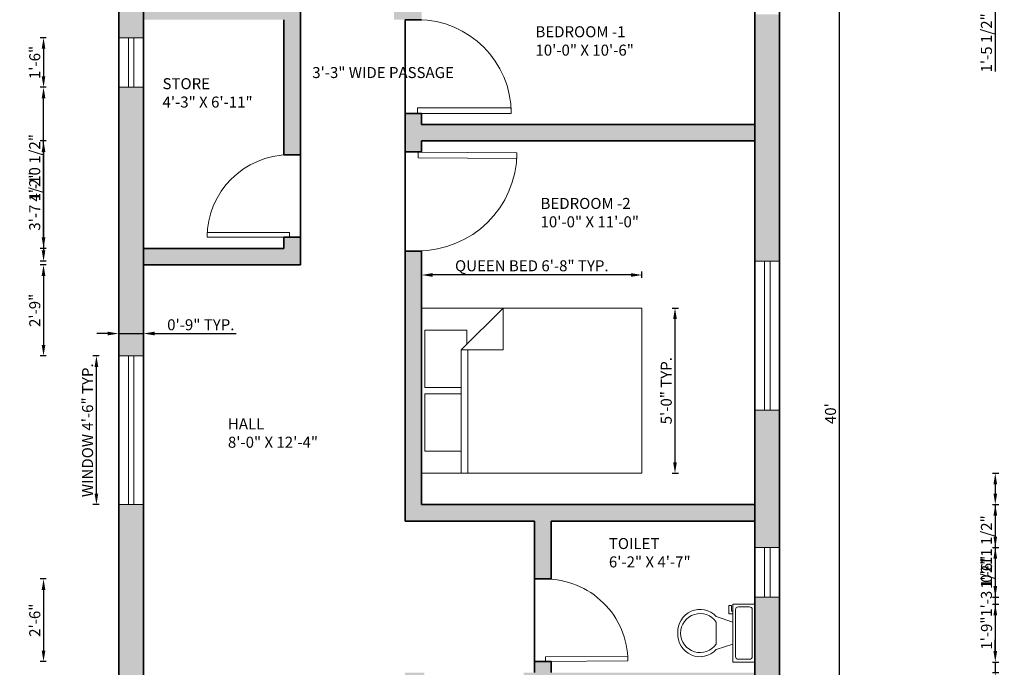
# Model space of a CAD drawing. Units: inches. Extents: x -35 to 322, y -513 to 50.
# Tile 2 of 3: x -35 to 322, y -318 to -83. Entities that reach past the tile are written whole.
import ezdxf

# ---------------------------------------------------------------- set-up
doc = ezdxf.new("R2010")
doc.units = ezdxf.units.IN
for name, color, linetype, lineweight in [('A-ANNO-DIMS', 2, 'Continuous', 18), ('A-AREA-IDEN', 7, 'Continuous', 18), ('A-DOOR', 4, 'Continuous', 18), ('A-FLOR-FIXT', 9, 'Continuous', 18), ('A-FURN', 8, 'Continuous', 18), ('A-GLAZ', 6, 'Continuous', 18), ('A-WALL', 7, 'Continuous', 35), ('A-WALL-PATT', 251, 'Continuous', 13)]:
    doc.layers.add(name, color=color, linetype=linetype, lineweight=lineweight)
doc.styles.get("Standard").update_dxf_attribs({"font": 'arial.ttf'})
doc.dimstyles.new('ISO-25', dxfattribs={"dimtxt": 4, "dimasz": 4, "dimexe": 1.25, "dimexo": 0.625, "dimtad": 1, "dimlunit": 3, "dimtxsty": 'Standard', "dimcen": 2.5, "dimadec": 0, "dimazin": 0, "dimtfac": 1, "dimtmove": 0, "dimatfit": 3, "dimfxl": 1, "dimfxlon": 1, "dimarcsym": 0})

# ---------------------------------------------------------------- blocks, each defined once
blk = doc.blocks.new('*U2')
for p, q in [((9.5, -6), (9.5, -2)), ((-10, -8.5), (-8, -8.5)), ((-10, -9.5), (-10, -8.5)), ((-7, -9.5), (-10, -9.5)), ((-8, -8.5), (-8, -8)), ((-7, -8), (-7, -9.5)), ((-4, -8), (-6, -14)), ((4, -8), (6, -14)), ((4, -14), (-4, -14))]:
    blk.add_line(p, q)
blk.add_lwpolyline([(10.5, -8), (10.5, 0), (-10.5, 0), (-10.5, -8)], close=True)
for points in [[(-9.5, -2), (-9.5, -6)], [(8.5, -1), (-8.5, -1)], [(-8.5, -7), (8.5, -7)]]:
    blk.add_lwpolyline(points)
for centre, radius, start, end in [((-8.625, -1.875), 0.8839, 81.8699, 188.1301), ((8.625, -1.875), 0.8839, 351.8699, 98.1301), ((-8.625, -6.125), 0.8839, 171.869898, 278.1301), ((8.625, -6.125), 0.8839, 261.8699, 8.1301), ((-0.4772, -19.9188), 8.0953, 133.01722, 273.38), ((0.0374, -19.8731), 7.127, 124.50543, 269.7), ((-0.0373, -19.8731), 7.127, 270.3, 55.4946), ((0.4773, -19.9188), 8.0953, 266.62, 46.9828)]:
    blk.add_arc(centre, radius, start, end)
blk = doc.blocks.new('*U4')
for p, q in [((0, 0), (0, -100)), ((750, 0), (750, -100))]:
    blk.add_line(p, q)
blk.add_lwpolyline([(0, 0), (0, 750), (43.75, 750), (43.75, 0)], close=True)
blk.add_arc((0, 0), 750, 0, 90)
blk = doc.blocks.new('Bed - Queen')
for p, q in [((0, -80.00003), (0, 0)), ((0, 0), (59.99999, 0)), ((59.99999, 0), (59.99999, -80.00003)), ((7.99999, -1.2), (28.79998, -1.2)), ((7.99999, -14.4), (7.99999, -1.2)), ((28.79998, -1.2), (28.79998, -14.4)), ((31.19999, -1.2), (51.99999, -1.2)), ((31.19999, -14.4), (31.19999, -1.2)), ((51.99999, -1.2), (51.99999, -16.4)), ((0, -14.4), (44.8, -14.4)), ((44.8, -16.8), (0, -16.8)), ((59.99999, -29.6), (44.8, -14.4)), ((44.8, -14.4), (44.8, -29.6)), ((51.99999, -16.4), (46.79936, -16.4)), ((44.8, -29.6), (59.99999, -29.6)), ((59.99999, -80.00003), (0, -80.00003))]:
    blk.add_line(p, q)
blk = doc.blocks.new('*D13')
at = {"layer": 'A-ANNO-DIMS', "color": 0, "lineweight": -2, "transparency": 16777216}
for p, q in [((261.29, 13.99), (263.54, 13.99)), ((262.29, 9.99), (262.29, -462.01)), ((261.29, -466.01), (263.54, -466.01))]:
    blk.add_line(p, q, dxfattribs=at)
at = {"layer": 'A-ANNO-DIMS', "color": 0, "transparency": 16777216}
for points in [[(261.62, 9.99), (262.95, 9.99), (262.29, 13.99)], [(261.62, -462.01), (262.95, -462.01), (262.29, -466.01)]]:
    blk.add_solid(points, dxfattribs=at)
at = {"layer": 'Defpoints', "color": 0, "transparency": 16777216}
for p in [(239.43, 13.99), (240.64, -466.01), (262.29, -466.01)]:
    blk.add_point(p, dxfattribs=at)
at = {"layer": 'A-ANNO-DIMS', "color": 0, "transparency": 16777216, "insert": (259.62, -226.01), "char_height": 4, "attachment_point": 5, "rotation": 90}
blk.add_mtext("40'", dxfattribs=at)
blk = doc.blocks.new('WIN-54IN')
for p, q in [((3.5, 54), (3.5, 0)), ((5.5, 54), (5.5, 0))]:
    blk.add_line(p, q)
blk.add_lwpolyline([(0, 54), (9, 54), (9, 0), (0, 0)], close=True)
blk = doc.blocks.new('*D16')
at = {"layer": 'A-ANNO-DIMS', "color": 0, "lineweight": -2, "transparency": 16777216}
for p, q in [((110.64, -176.68), (110.64, -174.43)), ((190.64, -176.68), (190.64, -174.43)), ((186.64, -175.68), (114.64, -175.68))]:
    blk.add_line(p, q, dxfattribs=at)
at = {"layer": 'A-ANNO-DIMS', "color": 0, "transparency": 16777216}
for points in [[(114.64, -175.01), (114.64, -176.35), (110.64, -175.68)], [(186.64, -175.01), (186.64, -176.35), (190.64, -175.68)]]:
    blk.add_solid(points, dxfattribs=at)
at = {"layer": 'Defpoints', "color": 0, "transparency": 16777216}
for p in [(110.64, -175.68), (110.64, -187.68), (190.64, -187.68)]:
    blk.add_point(p, dxfattribs=at)
at = {"layer": 'A-ANNO-DIMS', "color": 0, "transparency": 16777216, "insert": (150.64, -172.86), "char_height": 4, "attachment_point": 5}
blk.add_mtext('QUEEN BED 6\'-8" TYP.', dxfattribs=at)
blk = doc.blocks.new('*D17')
at = {"layer": 'A-ANNO-DIMS', "color": 0, "lineweight": -2, "transparency": 16777216}
for p, q in [((201.64, -187.68), (203.89, -187.68)), ((202.64, -243.68), (202.64, -191.68)), ((201.64, -247.68), (203.89, -247.68))]:
    blk.add_line(p, q, dxfattribs=at)
at = {"layer": 'A-ANNO-DIMS', "color": 0, "transparency": 16777216}
for points in [[(201.97, -191.68), (203.3, -191.68), (202.64, -187.68)], [(201.97, -243.68), (203.3, -243.68), (202.64, -247.68)]]:
    blk.add_solid(points, dxfattribs=at)
at = {"layer": 'Defpoints', "color": 0, "transparency": 16777216}
for p in [(190.64, -187.68), (202.64, -187.68), (190.64, -247.68)]:
    blk.add_point(p, dxfattribs=at)
at = {"layer": 'A-ANNO-DIMS', "color": 0, "transparency": 16777216, "insert": (199.97, -217.68), "char_height": 4, "attachment_point": 5, "rotation": 90}
blk.add_mtext('5\'-0" TYP.', dxfattribs=at)
blk = doc.blocks.new('*D18')
at = {"layer": 'A-ANNO-DIMS', "color": 0, "lineweight": -2, "transparency": 16777216}
for p, q in [((-6.46, -205.04), (-8.71, -205.04)), ((-7.46, -255.04), (-7.46, -209.04)), ((-6.46, -259.04), (-8.71, -259.04))]:
    blk.add_line(p, q, dxfattribs=at)
at = {"layer": 'A-ANNO-DIMS', "color": 0, "transparency": 16777216}
for points in [[(-8.13, -209.04), (-6.8, -209.04), (-7.46, -205.04)], [(-8.13, -255.04), (-6.8, -255.04), (-7.46, -259.04)]]:
    blk.add_solid(points, dxfattribs=at)
at = {"layer": 'Defpoints', "color": 0, "transparency": 16777216}
for p in [(-7.46, -205.04), (0.64, -205.04), (0.64, -259.04)]:
    blk.add_point(p, dxfattribs=at)
at = {"layer": 'A-ANNO-DIMS', "color": 0, "transparency": 16777216, "insert": (-10.16, -232.04), "char_height": 4, "attachment_point": 5, "rotation": 90}
blk.add_mtext('WINDOW 4\'-6" TYP.', dxfattribs=at)
blk = doc.blocks.new('*D19')
at = {"layer": 'A-ANNO-DIMS', "color": 0, "lineweight": -2, "transparency": 16777216}
for p, q in [((0.64, -197.94), (0.64, -195.69)), ((9.64, -197.94), (9.64, -195.69)), ((-3.36, -196.94), (-7.36, -196.94)), ((0.64, -196.94), (9.64, -196.94)), ((13.64, -196.94), (43.27, -196.94))]:
    blk.add_line(p, q, dxfattribs=at)
at = {"layer": 'A-ANNO-DIMS', "color": 0, "transparency": 16777216}
for points in [[(-3.36, -196.27), (-3.36, -197.61), (0.64, -196.94)], [(13.64, -196.27), (13.64, -197.61), (9.64, -196.94)]]:
    blk.add_solid(points, dxfattribs=at)
at = {"layer": 'Defpoints', "color": 0, "transparency": 16777216}
for p in [(9.64, -196.94), (0.64, -205.04), (9.64, -205.04)]:
    blk.add_point(p, dxfattribs=at)
at = {"layer": 'A-ANNO-DIMS', "color": 0, "transparency": 16777216, "insert": (30.45, -194.27), "char_height": 4, "attachment_point": 5}
blk.add_mtext('0\'-9" TYP.', dxfattribs=at)
blk = doc.blocks.new('*D26')
at = {"layer": 'A-ANNO-DIMS', "color": 0, "lineweight": -2, "transparency": 16777216}
for p, q in [((100.64, -509.7), (96.64, -509.7)), ((104.64, -508.7), (104.64, -510.95)), ((104.64, -509.7), (110.64, -509.7)), ((110.64, -508.7), (110.64, -510.95)), ((114.64, -509.7), (130.52, -509.7))]:
    blk.add_line(p, q, dxfattribs=at)
at = {"layer": 'A-ANNO-DIMS', "color": 0, "transparency": 16777216}
for points in [[(100.64, -509.04), (100.64, -510.37), (104.64, -509.7)], [(114.64, -509.04), (114.64, -510.37), (110.64, -509.7)]]:
    blk.add_solid(points, dxfattribs=at)
at = {"layer": 'Defpoints', "color": 0, "transparency": 16777216}
for p in [(104.64, -77.01), (110.64, -83.01), (110.64, -509.7)]:
    blk.add_point(p, dxfattribs=at)
at = {"layer": 'A-ANNO-DIMS', "color": 0, "transparency": 16777216, "insert": (124.58, -507.04), "char_height": 4, "attachment_point": 5}
blk.add_mtext('0\'-6"', dxfattribs=at)
blk = doc.blocks.new('*D29')
at = {"layer": 'A-ANNO-DIMS', "color": 0, "lineweight": -2, "transparency": 16777216}
for p, q in [((66.64, 40.29), (66.64, 42.54)), ((70.64, 41.29), (100.64, 41.29)), ((104.64, 40.29), (104.64, 42.54))]:
    blk.add_line(p, q, dxfattribs=at)
at = {"layer": 'A-ANNO-DIMS', "color": 0, "transparency": 16777216}
for points in [[(70.64, 41.95), (70.64, 40.62), (66.64, 41.29)], [(100.64, 41.95), (100.64, 40.62), (104.64, 41.29)]]:
    blk.add_solid(points, dxfattribs=at)
at = {"layer": 'Defpoints', "color": 0, "transparency": 16777216}
for p in [(104.64, 41.29), (66.64, -466.01), (104.64, -466.01)]:
    blk.add_point(p, dxfattribs=at)
at = {"layer": 'A-ANNO-DIMS', "color": 0, "transparency": 16777216, "insert": (85.64, 43.96), "char_height": 4, "attachment_point": 5}
blk.add_mtext('3\'-2"', dxfattribs=at)
blk = doc.blocks.new('*D35')
at = {"layer": 'A-ANNO-DIMS', "color": 0, "lineweight": -2, "transparency": 16777216}
for p, q in [((-25.66, -107.55), (-27.91, -107.55)), ((-26.66, -162.01), (-26.66, -111.55)), ((-25.66, -166.01), (-27.91, -166.01))]:
    blk.add_line(p, q, dxfattribs=at)
at = {"layer": 'A-ANNO-DIMS', "color": 0, "transparency": 16777216}
for points in [[(-27.33, -111.55), (-26, -111.55), (-26.66, -107.55)], [(-27.33, -162.01), (-26, -162.01), (-26.66, -166.01)]]:
    blk.add_solid(points, dxfattribs=at)
at = {"layer": 'Defpoints', "color": 0, "transparency": 16777216}
for p in [(-26.66, -107.55), (9.64, -107.55), (9.64, -166.01)]:
    blk.add_point(p, dxfattribs=at)
at = {"layer": 'A-ANNO-DIMS', "color": 0, "transparency": 16777216, "insert": (-29.36, -136.78), "char_height": 4, "attachment_point": 5, "rotation": 90}
blk.add_mtext('4\'-10 1/2"', dxfattribs=at)
blk = doc.blocks.new('*D36')
at = {"layer": 'A-ANNO-DIMS', "color": 0, "lineweight": -2, "transparency": 16777216}
for p, q in [((-25.66, -89.55), (-27.91, -89.55)), ((-26.66, -93.55), (-26.66, -103.55)), ((-25.66, -107.55), (-27.91, -107.55))]:
    blk.add_line(p, q, dxfattribs=at)
at = {"layer": 'A-ANNO-DIMS', "color": 0, "transparency": 16777216}
for points in [[(-27.33, -93.55), (-26, -93.55), (-26.66, -89.55)], [(-27.33, -103.55), (-26, -103.55), (-26.66, -107.55)]]:
    blk.add_solid(points, dxfattribs=at)
at = {"layer": 'Defpoints', "color": 0, "transparency": 16777216}
for p in [(0.64, -89.55), (-26.66, -107.55), (0.64, -107.55)]:
    blk.add_point(p, dxfattribs=at)
at = {"layer": 'A-ANNO-DIMS', "color": 0, "transparency": 16777216, "insert": (-29.33, -98.55), "char_height": 4, "attachment_point": 5, "rotation": 90}
blk.add_mtext('1\'-6"', dxfattribs=at)
blk = doc.blocks.new('*D37')
at = {"layer": 'A-ANNO-DIMS', "color": 0, "lineweight": -2, "transparency": 16777216}
for p, q in [((-25.66, -172.01), (-27.91, -172.01)), ((-26.66, -176.01), (-26.66, -201.04)), ((-25.66, -205.04), (-27.91, -205.04))]:
    blk.add_line(p, q, dxfattribs=at)
at = {"layer": 'A-ANNO-DIMS', "color": 0, "transparency": 16777216}
for points in [[(-27.33, -176.01), (-26, -176.01), (-26.66, -172.01)], [(-27.33, -201.04), (-26, -201.04), (-26.66, -205.04)]]:
    blk.add_solid(points, dxfattribs=at)
at = {"layer": 'Defpoints', "color": 0, "transparency": 16777216}
for p in [(9.64, -172.01), (-26.66, -205.04), (9.64, -205.04)]:
    blk.add_point(p, dxfattribs=at)
at = {"layer": 'A-ANNO-DIMS', "color": 0, "transparency": 16777216, "insert": (-29.33, -188.53), "char_height": 4, "attachment_point": 5, "rotation": 90}
blk.add_mtext('2\'-9"', dxfattribs=at)
blk = doc.blocks.new('*D39')
at = {"layer": 'A-ANNO-DIMS', "color": 0, "lineweight": -2, "transparency": 16777216}
for p, q in [((-25.66, -127.01), (-27.91, -127.01)), ((-26.66, -131.01), (-26.66, -166.72)), ((-25.66, -170.72), (-27.91, -170.72))]:
    blk.add_line(p, q, dxfattribs=at)
at = {"layer": 'A-ANNO-DIMS', "color": 0, "transparency": 16777216}
for points in [[(-27.33, -131.01), (-26, -131.01), (-26.66, -127.01)], [(-27.33, -166.72), (-26, -166.72), (-26.66, -170.72)]]:
    blk.add_solid(points, dxfattribs=at)
at = {"layer": 'Defpoints', "color": 0, "transparency": 16777216}
for p in [(231.64, -127.01), (-26.66, -170.72), (231.64, -170.72)]:
    blk.add_point(p, dxfattribs=at)
at = {"layer": 'A-ANNO-DIMS', "color": 0, "transparency": 16777216, "insert": (-29.36, -148.86), "char_height": 4, "attachment_point": 5, "rotation": 90}
blk.add_mtext('3\'-7 1/2"', dxfattribs=at)
blk = doc.blocks.new('*D40')
at = {"layer": 'A-ANNO-DIMS', "color": 0, "lineweight": -2, "transparency": 16777216}
for p, q in [((317.94, -259.01), (320.19, -259.01)), ((318.94, -263.01), (318.94, -270.62)), ((317.94, -274.62), (320.19, -274.62)), ((318.94, -274.62), (318.94, -299.45))]:
    blk.add_line(p, q, dxfattribs=at)
at = {"layer": 'A-ANNO-DIMS', "color": 0, "transparency": 16777216}
for points in [[(318.27, -263.01), (319.6, -263.01), (318.94, -259.01)], [(318.27, -270.62), (319.6, -270.62), (318.94, -274.62)]]:
    blk.add_solid(points, dxfattribs=at)
at = {"layer": 'Defpoints', "color": 0, "transparency": 16777216}
for p in [(231.64, -259.01), (240.64, -274.62), (318.94, -274.62)]:
    blk.add_point(p, dxfattribs=at)
at = {"layer": 'A-ANNO-DIMS', "color": 0, "transparency": 16777216, "insert": (316.24, -289.04), "char_height": 4, "attachment_point": 5, "rotation": 90}
blk.add_mtext('1\'-3 1/2"', dxfattribs=at)
blk = doc.blocks.new('*D41')
at = {"layer": 'A-ANNO-DIMS', "color": 0, "lineweight": -2, "transparency": 16777216}
for p, q in [((317.94, -274.62), (320.19, -274.62)), ((318.94, -278.62), (318.94, -288.62)), ((317.94, -292.62), (320.19, -292.62))]:
    blk.add_line(p, q, dxfattribs=at)
at = {"layer": 'A-ANNO-DIMS', "color": 0, "transparency": 16777216}
for points in [[(318.27, -278.62), (319.6, -278.62), (318.94, -274.62)], [(318.27, -288.62), (319.6, -288.62), (318.94, -292.62)]]:
    blk.add_solid(points, dxfattribs=at)
at = {"layer": 'Defpoints', "color": 0, "transparency": 16777216}
for p in [(240.64, -274.62), (240.64, -292.62), (318.94, -292.62)]:
    blk.add_point(p, dxfattribs=at)
at = {"layer": 'A-ANNO-DIMS', "color": 0, "transparency": 16777216, "insert": (316.27, -283.62), "char_height": 4, "attachment_point": 5, "rotation": 90}
blk.add_mtext('1\'-6"', dxfattribs=at)
blk = doc.blocks.new('*D42')
at = {"layer": 'A-ANNO-DIMS', "color": 0, "lineweight": -2, "transparency": 16777216}
for p, q in [((196.08, 40.29), (196.08, 42.54)), ((200.08, 41.29), (227.64, 41.29)), ((231.64, 40.29), (231.64, 42.54))]:
    blk.add_line(p, q, dxfattribs=at)
at = {"layer": 'A-ANNO-DIMS', "color": 0, "transparency": 16777216}
for points in [[(200.08, 41.95), (200.08, 40.62), (196.08, 41.29)], [(227.64, 41.95), (227.64, 40.62), (231.64, 41.29)]]:
    blk.add_solid(points, dxfattribs=at)
at = {"layer": 'Defpoints', "color": 0, "transparency": 16777216}
for p in [(231.64, 41.29), (196.08, -457.01), (231.64, -457.01)]:
    blk.add_point(p, dxfattribs=at)
at = {"layer": 'A-ANNO-DIMS', "color": 0, "transparency": 16777216, "insert": (213.86, 43.98), "char_height": 4, "attachment_point": 5}
blk.add_mtext('2\'-11 1/2"', dxfattribs=at)
blk = doc.blocks.new('*D43')
at = {"layer": 'A-ANNO-DIMS', "color": 0, "lineweight": -2, "transparency": 16777216}
for p, q in [((66.64, -508.7), (66.64, -510.95)), ((70.64, -509.7), (96.64, -509.7)), ((100.64, -508.7), (100.64, -510.95))]:
    blk.add_line(p, q, dxfattribs=at)
at = {"layer": 'A-ANNO-DIMS', "color": 0, "transparency": 16777216}
for points in [[(70.64, -509.04), (70.64, -510.37), (66.64, -509.7)], [(96.64, -509.04), (96.64, -510.37), (100.64, -509.7)]]:
    blk.add_solid(points, dxfattribs=at)
at = {"layer": 'Defpoints', "color": 0, "transparency": 16777216}
for p in [(66.64, -83.01), (100.64, -83.01), (100.64, -509.7)]:
    blk.add_point(p, dxfattribs=at)
at = {"layer": 'A-ANNO-DIMS', "color": 0, "transparency": 16777216, "insert": (83.64, -507.04), "char_height": 4, "attachment_point": 5}
blk.add_mtext('2\'-10"', dxfattribs=at)
blk = doc.blocks.new('*D46')
at = {"layer": 'A-ANNO-DIMS', "color": 0, "lineweight": -2, "transparency": 16777216}
for p, q in [((32.73, 40.29), (32.73, 42.54)), ((36.73, 41.29), (58.65, 41.29)), ((62.65, 40.29), (62.65, 42.54))]:
    blk.add_line(p, q, dxfattribs=at)
at = {"layer": 'A-ANNO-DIMS', "color": 0, "transparency": 16777216}
for points in [[(36.73, 41.95), (36.73, 40.62), (32.73, 41.29)], [(58.65, 41.95), (58.65, 40.62), (62.65, 41.29)]]:
    blk.add_solid(points, dxfattribs=at)
at = {"layer": 'Defpoints', "color": 0, "transparency": 16777216}
for p in [(62.65, 41.29), (32.73, -162.01), (62.65, -162.01)]:
    blk.add_point(p, dxfattribs=at)
at = {"layer": 'A-ANNO-DIMS', "color": 0, "transparency": 16777216, "insert": (47.69, 43.95), "char_height": 4, "attachment_point": 5}
blk.add_mtext('2\'-6"', dxfattribs=at)
blk = doc.blocks.new('*D47')
at = {"layer": 'A-ANNO-DIMS', "color": 0, "lineweight": -2, "transparency": 16777216}
for p, q in [((109.17, 40.29), (109.17, 42.54)), ((113.17, 41.29), (139.16, 41.29)), ((143.16, 40.29), (143.16, 42.54))]:
    blk.add_line(p, q, dxfattribs=at)
at = {"layer": 'A-ANNO-DIMS', "color": 0, "transparency": 16777216}
for points in [[(113.17, 41.95), (113.17, 40.62), (109.17, 41.29)], [(139.16, 41.95), (139.16, 40.62), (143.16, 41.29)]]:
    blk.add_solid(points, dxfattribs=at)
at = {"layer": 'Defpoints', "color": 0, "transparency": 16777216}
for p in [(143.16, 41.29), (109.17, -117.01), (143.16, -117.01)]:
    blk.add_point(p, dxfattribs=at)
at = {"layer": 'A-ANNO-DIMS', "color": 0, "transparency": 16777216, "insert": (126.17, 43.95), "char_height": 4, "attachment_point": 5}
blk.add_mtext('2\'-10"', dxfattribs=at)
blk = doc.blocks.new('*D48')
at = {"layer": 'A-ANNO-DIMS', "color": 0, "lineweight": -2, "transparency": 16777216}
for p, q in [((109.42, -508.7), (109.42, -510.95)), ((113.42, -509.7), (141.25, -509.7)), ((145.25, -508.7), (145.25, -510.95))]:
    blk.add_line(p, q, dxfattribs=at)
at = {"layer": 'A-ANNO-DIMS', "color": 0, "transparency": 16777216}
for points in [[(113.42, -509.04), (113.42, -510.37), (109.42, -509.7)], [(141.25, -509.04), (141.25, -510.37), (145.25, -509.7)]]:
    blk.add_solid(points, dxfattribs=at)
at = {"layer": 'Defpoints', "color": 0, "transparency": 16777216}
for p in [(109.42, -131.05), (145.25, -131.34), (145.25, -509.7)]:
    blk.add_point(p, dxfattribs=at)
at = {"layer": 'A-ANNO-DIMS', "color": 0, "transparency": 16777216, "insert": (127.34, -507.04), "char_height": 4, "attachment_point": 5}
blk.add_mtext('3\'-0"', dxfattribs=at)
blk = doc.blocks.new('*D49')
at = {"layer": 'A-ANNO-DIMS', "color": 0, "lineweight": -2, "transparency": 16777216}
for p, q in [((-25.66, -286.01), (-27.91, -286.01)), ((-26.66, -290.01), (-26.66, -312.01)), ((-25.66, -316.01), (-27.91, -316.01))]:
    blk.add_line(p, q, dxfattribs=at)
at = {"layer": 'A-ANNO-DIMS', "color": 0, "transparency": 16777216}
for points in [[(-27.33, -290.01), (-26, -290.01), (-26.66, -286.01)], [(-27.33, -312.01), (-26, -312.01), (-26.66, -316.01)]]:
    blk.add_solid(points, dxfattribs=at)
at = {"layer": 'Defpoints', "color": 0, "transparency": 16777216}
for p in [(151.64, -286.01), (-26.66, -316.01), (151.64, -316.01)]:
    blk.add_point(p, dxfattribs=at)
at = {"layer": 'A-ANNO-DIMS', "color": 0, "transparency": 16777216, "insert": (-29.33, -301.01), "char_height": 4, "attachment_point": 5, "rotation": 90}
blk.add_mtext('2\'-6"', dxfattribs=at)
blk = doc.blocks.new('*D50')
at = {"layer": 'A-ANNO-DIMS', "color": 0, "lineweight": -2, "transparency": 16777216}
for p, q in [((111.64, 40.29), (111.64, 42.54)), ((115.64, 41.29), (143.64, 41.29)), ((147.64, 40.29), (147.64, 42.54))]:
    blk.add_line(p, q, dxfattribs=at)
at = {"layer": 'A-ANNO-DIMS', "color": 0, "transparency": 16777216}
for points in [[(115.64, 41.95), (115.64, 40.62), (111.64, 41.29)], [(143.64, 41.95), (143.64, 40.62), (147.64, 41.29)]]:
    blk.add_solid(points, dxfattribs=at)
at = {"layer": 'Defpoints', "color": 0, "transparency": 16777216}
for p in [(147.64, 41.29), (111.64, -320.01), (147.64, -320.01)]:
    blk.add_point(p, dxfattribs=at)
at = {"layer": 'A-ANNO-DIMS', "color": 0, "transparency": 16777216, "insert": (129.64, 43.96), "char_height": 4, "attachment_point": 5}
blk.add_mtext('3\'-0"', dxfattribs=at)
blk = doc.blocks.new('*D51')
at = {"layer": 'A-ANNO-DIMS', "color": 0, "lineweight": -2, "transparency": 16777216}
for p, q in [((203.64, 40.29), (203.64, 42.54)), ((207.64, 41.29), (227.64, 41.29)), ((231.64, 40.29), (231.64, 42.54))]:
    blk.add_line(p, q, dxfattribs=at)
at = {"layer": 'A-ANNO-DIMS', "color": 0, "transparency": 16777216}
for points in [[(207.64, 41.95), (207.64, 40.62), (203.64, 41.29)], [(227.64, 41.95), (227.64, 40.62), (231.64, 41.29)]]:
    blk.add_solid(points, dxfattribs=at)
at = {"layer": 'Defpoints', "color": 0, "transparency": 16777216}
for p in [(231.64, 41.29), (231.64, -295.18), (203.64, -305.68)]:
    blk.add_point(p, dxfattribs=at)
at = {"layer": 'A-ANNO-DIMS', "color": 0, "transparency": 16777216, "insert": (217.64, 43.92), "char_height": 4, "attachment_point": 5}
blk.add_mtext('2\'-4"', dxfattribs=at)
blk = doc.blocks.new('*D52')
at = {"layer": 'A-ANNO-DIMS', "color": 0, "lineweight": -2, "transparency": 16777216}
for p, q in [((317.94, -295.18), (320.19, -295.18)), ((318.94, -299.18), (318.94, -312.18)), ((317.94, -316.18), (320.19, -316.18))]:
    blk.add_line(p, q, dxfattribs=at)
at = {"layer": 'A-ANNO-DIMS', "color": 0, "transparency": 16777216}
for points in [[(318.27, -299.18), (319.6, -299.18), (318.94, -295.18)], [(318.27, -312.18), (319.6, -312.18), (318.94, -316.18)]]:
    blk.add_solid(points, dxfattribs=at)
at = {"layer": 'Defpoints', "color": 0, "transparency": 16777216}
for p in [(231.64, -295.18), (231.64, -316.18), (318.94, -316.18)]:
    blk.add_point(p, dxfattribs=at)
at = {"layer": 'A-ANNO-DIMS', "color": 0, "transparency": 16777216, "insert": (316.27, -305.68), "char_height": 4, "attachment_point": 5, "rotation": 90}
blk.add_mtext('1\'-9"', dxfattribs=at)
blk = doc.blocks.new('*D53')
at = {"layer": 'A-ANNO-DIMS', "color": 0, "lineweight": -2, "transparency": 16777216}
for p, q in [((318.94, -312.18), (318.94, -308.18)), ((317.94, -316.18), (320.19, -316.18)), ((318.94, -316.18), (318.94, -320.01)), ((317.94, -320.01), (320.19, -320.01)), ((318.94, -324.01), (318.94, -339.9))]:
    blk.add_line(p, q, dxfattribs=at)
at = {"layer": 'A-ANNO-DIMS', "color": 0, "transparency": 16777216}
for points in [[(318.27, -312.18), (319.6, -312.18), (318.94, -316.18)], [(318.27, -324.01), (319.6, -324.01), (318.94, -320.01)]]:
    blk.add_solid(points, dxfattribs=at)
at = {"layer": 'Defpoints', "color": 0, "transparency": 16777216}
for p in [(231.64, -316.18), (231.64, -320.01), (318.94, -320.01)]:
    blk.add_point(p, dxfattribs=at)
at = {"layer": 'A-ANNO-DIMS', "color": 0, "transparency": 16777216, "insert": (316.27, -333.95), "char_height": 4, "attachment_point": 5, "rotation": 90}
blk.add_mtext('0\'-4"', dxfattribs=at)
blk = doc.blocks.new('*D54')
at = {"layer": 'A-ANNO-DIMS', "color": 0, "lineweight": -2, "transparency": 16777216}
for p, q in [((209.06, -508.7), (209.06, -510.95)), ((213.06, -509.7), (227.64, -509.7)), ((231.64, -508.7), (231.64, -510.95)), ((231.64, -509.7), (259.57, -509.7))]:
    blk.add_line(p, q, dxfattribs=at)
at = {"layer": 'A-ANNO-DIMS', "color": 0, "transparency": 16777216}
for points in [[(213.06, -509.04), (213.06, -510.37), (209.06, -509.7)], [(227.64, -509.04), (227.64, -510.37), (231.64, -509.7)]]:
    blk.add_solid(points, dxfattribs=at)
at = {"layer": 'Defpoints', "color": 0, "transparency": 16777216}
for p in [(209.06, 4.99), (231.64, 4.99), (231.64, -509.7)]:
    blk.add_point(p, dxfattribs=at)
at = {"layer": 'A-ANNO-DIMS', "color": 0, "transparency": 16777216, "insert": (247.6, -507.01), "char_height": 4, "attachment_point": 5}
blk.add_mtext('1\'-10 1/2"', dxfattribs=at)
blk = doc.blocks.new('*D55')
at = {"layer": 'A-ANNO-DIMS', "color": 0, "lineweight": -2, "transparency": 16777216}
for p, q in [((317.94, -247.68), (320.19, -247.68)), ((318.94, -251.68), (318.94, -255.01)), ((317.94, -259.01), (320.19, -259.01)), ((318.94, -259.01), (318.94, -287.32))]:
    blk.add_line(p, q, dxfattribs=at)
at = {"layer": 'A-ANNO-DIMS', "color": 0, "transparency": 16777216}
for points in [[(318.27, -251.68), (319.6, -251.68), (318.94, -247.68)], [(318.27, -255.01), (319.6, -255.01), (318.94, -259.01)]]:
    blk.add_solid(points, dxfattribs=at)
at = {"layer": 'Defpoints', "color": 0, "transparency": 16777216}
for p in [(190.64, -247.68), (231.64, -259.01), (318.94, -259.01)]:
    blk.add_point(p, dxfattribs=at)
at = {"layer": 'A-ANNO-DIMS', "color": 0, "transparency": 16777216, "insert": (316.24, -275.17), "char_height": 4, "attachment_point": 5, "rotation": 90}
blk.add_mtext('0\'-11 1/2"', dxfattribs=at)
blk = doc.blocks.new('*D59')
at = {"layer": 'A-ANNO-DIMS', "color": 0, "lineweight": -2, "transparency": 16777216}
for p, q in [((317.94, -59.34), (320.19, -59.34)), ((318.94, -63.34), (318.94, -73.01)), ((317.94, -77.01), (320.19, -77.01)), ((318.94, -77.01), (318.94, -101.84))]:
    blk.add_line(p, q, dxfattribs=at)
at = {"layer": 'A-ANNO-DIMS', "color": 0, "transparency": 16777216}
for points in [[(318.27, -63.34), (319.6, -63.34), (318.94, -59.34)], [(318.27, -73.01), (319.6, -73.01), (318.94, -77.01)]]:
    blk.add_solid(points, dxfattribs=at)
at = {"layer": 'Defpoints', "color": 0, "transparency": 16777216}
for p in [(29.69, -59.34), (33.64, -77.01), (318.94, -77.01)]:
    blk.add_point(p, dxfattribs=at)
at = {"layer": 'A-ANNO-DIMS', "color": 0, "transparency": 16777216, "insert": (316.24, -91.43), "char_height": 4, "attachment_point": 5, "rotation": 90}
blk.add_mtext('1\'-5 1/2"', dxfattribs=at)
blk = doc.blocks.new('*D61')
at = {"layer": 'A-ANNO-DIMS', "color": 0, "lineweight": -2, "transparency": 16777216}
for p, q in [((35.64, 41.29), (31.64, 41.29)), ((39.64, 40.29), (39.64, 42.54)), ((39.64, 41.29), (46.39, 41.29)), ((46.39, 40.29), (46.39, 42.54)), ((50.39, 41.29), (66.27, 41.29))]:
    blk.add_line(p, q, dxfattribs=at)
at = {"layer": 'A-ANNO-DIMS', "color": 0, "transparency": 16777216}
for points in [[(35.64, 41.95), (35.64, 40.62), (39.64, 41.29)], [(50.39, 41.95), (50.39, 40.62), (46.39, 41.29)]]:
    blk.add_solid(points, dxfattribs=at)
at = {"layer": 'Defpoints', "color": 0, "transparency": 16777216}
for p in [(46.39, 41.29), (39.64, -326.01), (46.39, -326.01)]:
    blk.add_point(p, dxfattribs=at)
at = {"layer": 'A-ANNO-DIMS', "color": 0, "transparency": 16777216, "insert": (60.33, 43.95), "char_height": 4, "attachment_point": 5}
blk.add_mtext('0\'-7"', dxfattribs=at)

msp = doc.modelspace()

# ---------------------------------------------------------------- hatches: boundary and pattern name
at = {"layer": 'A-WALL-PATT'}
h = msp.add_hatch(color=256, dxfattribs=at)
h.dxf.hatch_style = 1
h.paths.add_polyline_path([(63.099, 13.987), (0.637, 13.987), (0.637, -26.079), (9.637, -26.079), (9.637, 4.987), (63.099, 4.987)])
h.paths.add_polyline_path([(9.637, -107.554), (0.637, -107.554), (0.637, -205.04), (9.637, -205.04)])
h.paths.add_polyline_path([(9.637, -60.079), (0.637, -60.079), (0.637, -89.554), (9.637, -89.554)])
h.paths.add_polyline_path([(9.637, -259.04), (0.637, -259.04), (0.637, -466.013), (66.468, -466.013), (66.468, -460.924, -0.0235925), (66.637, -457.328), (66.637, -457.013), (9.637, -457.013), (9.637, -326.013)])
h.paths.add_polyline_path([(142.082, -457.013), (104.637, -457.013), (104.637, -460.924), (104.637, -466.013), (142.082, -466.013)])
h.paths.add_polyline_path([(240.637, -224.716), (231.637, -224.716), (231.637, -274.623), (240.637, -274.623)])
h.paths.add_polyline_path([(69.474, -113.132), (98.939, -113.132), (98.939, -98.154), (69.474, -98.154)], flags=9)
h.paths.add_polyline_path([(38.843, -240.589), (73.258, -240.589), (73.258, -225.663), (38.843, -225.663)], flags=9)
h.paths.add_polyline_path([(51.03, -393.995), (85.248, -393.995), (85.248, -379.069), (51.03, -379.069)], flags=9)
h.paths.add_polyline_path([(75.428, -462.589), (96.367, -462.589), (96.367, -454.346), (75.428, -454.346)], flags=9)
h.paths.add_polyline_path([(154.313, -353.536), (191.907, -353.536), (191.907, -338.61), (154.313, -338.61)], flags=9)
h.paths.add_polyline_path([(177.411, -284.106), (208.497, -284.106), (208.497, -269.18), (177.411, -269.18)], flags=9)
h.paths.add_polyline_path([(152.205, -160.654), (189.798, -160.654), (189.798, -145.728), (152.205, -145.728)], flags=9)
h.paths.add_polyline_path([(150.351, -98.334), (187.945, -98.334), (187.945, -83.408), (150.351, -83.408)], flags=9)
h.paths.add_polyline_path([(15.293, -117.178), (49.667, -117.178), (49.667, -102.252), (15.293, -102.252)], flags=9)
h.paths.add_polyline_path([(40.377, -44.483), (77.823, -44.483), (77.823, -29.557), (40.377, -29.557)], flags=9)
h.paths.add_polyline_path([(31.67, -336.447), (44.796, -336.447), (44.796, -328.204), (31.67, -328.204)], flags=25)
h = msp.add_hatch(color=256, dxfattribs=at)
h.dxf.hatch_style = 1
h.paths.add_polyline_path([(110.637, -167.013), (104.637, -167.013), (104.637, -265.013), (151.637, -265.013), (151.637, -286.013), (157.637, -286.013), (157.637, -265.013), (231.637, -265.013), (231.637, -259.013), (110.637, -259.013)])
h.paths.add_polyline_path([(240.637, 13.987), (81.099, 13.987), (81.099, 4.987), (104.637, 4.987), (110.637, 4.987), (231.637, 4.987), (231.637, -27.021), (240.637, -27.021)])
h = msp.add_hatch(color=256, dxfattribs=at)
h.dxf.hatch_style = 1
h.paths.add_polyline_path([(110.637, 4.987), (104.637, 4.987), (104.637, -77.013), (100.637, -77.013), (100.637, -78.48), (100.637, -83.013), (104.637, -83.013), (110.637, -83.013)])
h.paths.add_polyline_path([(231.637, -121.013), (110.637, -121.013), (110.637, -117.013), (109.17, -117.013), (104.637, -117.013), (104.637, -131.013), (110.637, -131.013), (110.637, -127.013), (231.637, -127.013)])
h.paths.add_polyline_path([(15.293, -117.178), (49.667, -117.178), (49.667, -102.252), (15.293, -102.252)], flags=9)
h.paths.add_polyline_path([(69.474, -113.132), (98.939, -113.132), (98.939, -98.154), (69.474, -98.154)], flags=9)
h.paths.add_polyline_path([(38.843, -240.589), (73.258, -240.589), (73.258, -225.663), (38.843, -225.663)], flags=9)
h.paths.add_polyline_path([(51.03, -393.995), (85.248, -393.995), (85.248, -379.069), (51.03, -379.069)], flags=9)
h.paths.add_polyline_path([(75.428, -462.589), (96.367, -462.589), (96.367, -454.346), (75.428, -454.346)], flags=9)
h.paths.add_polyline_path([(154.313, -353.536), (191.907, -353.536), (191.907, -338.61), (154.313, -338.61)], flags=9)
h.paths.add_polyline_path([(177.411, -284.106), (208.497, -284.106), (208.497, -269.18), (177.411, -269.18)], flags=9)
h.paths.add_polyline_path([(152.205, -160.654), (189.798, -160.654), (189.798, -145.728), (152.205, -145.728)], flags=9)
h.paths.add_polyline_path([(150.351, -98.334), (187.945, -98.334), (187.945, -83.408), (150.351, -83.408)], flags=9)
h.paths.add_polyline_path([(40.377, -44.483), (77.823, -44.483), (77.823, -29.557), (40.377, -29.557)], flags=9)
h = msp.add_hatch(color=256, dxfattribs=at)
h.dxf.hatch_style = 1
h.paths.add_polyline_path([(110.637, -326.013), (111.637, -326.013), (111.637, -324.8), (111.637, -320.013), (104.637, -320.013), (104.637, -457.013), (110.637, -457.013)])
h.paths.add_polyline_path([(231.637, -320.013), (157.637, -320.013), (157.637, -316.013), (153.631, -316.013), (151.637, -316.029), (151.637, -320.013), (147.637, -320.013), (147.637, -326.013), (151.637, -326.013), (157.637, -326.013), (231.637, -326.013)])
h.paths.add_polyline_path([(240.637, -292.623), (231.637, -292.623), (231.637, -457.013), (196.082, -457.013), (196.082, -466.013), (240.637, -466.013)])
h.paths.add_polyline_path([(15.293, -117.178), (49.667, -117.178), (49.667, -102.252), (15.293, -102.252)], flags=9)
h.paths.add_polyline_path([(69.474, -113.132), (98.939, -113.132), (98.939, -98.154), (69.474, -98.154)], flags=9)
h.paths.add_polyline_path([(38.843, -240.589), (73.258, -240.589), (73.258, -225.663), (38.843, -225.663)], flags=9)
h.paths.add_polyline_path([(51.03, -393.995), (85.248, -393.995), (85.248, -379.069), (51.03, -379.069)], flags=9)
h.paths.add_polyline_path([(75.428, -462.589), (96.367, -462.589), (96.367, -454.346), (75.428, -454.346)], flags=9)
h.paths.add_polyline_path([(154.313, -353.536), (191.907, -353.536), (191.907, -338.61), (154.313, -338.61)], flags=9)
h.paths.add_polyline_path([(152.205, -160.654), (189.798, -160.654), (189.798, -145.728), (152.205, -145.728)], flags=9)
h.paths.add_polyline_path([(150.351, -98.334), (187.945, -98.334), (187.945, -83.408), (150.351, -83.408)], flags=9)
h.paths.add_polyline_path([(40.377, -44.483), (77.823, -44.483), (77.823, -29.557), (40.377, -29.557)], flags=9)
h = msp.add_hatch(color=256, dxfattribs=at)
h.dxf.hatch_style = 1
h.paths.add_polyline_path([(66.637, -77.013), (9.637, -77.013), (9.637, -83.013), (60.637, -83.013), (60.637, -132.013), (66.637, -132.013), (66.637, -83.013), (66.636, -78.48)])
h.paths.add_polyline_path([(66.637, -162.013), (62.648, -162.013), (60.637, -162.013), (60.637, -166.013), (9.637, -166.013), (9.637, -172.013), (60.637, -172.013), (66.637, -172.013)])
h = msp.add_hatch(color=256, dxfattribs=at)
h.dxf.hatch_style = 1
h.paths.add_polyline_path([(240.637, -81.021), (231.637, -81.021), (231.637, -170.716), (240.637, -170.716)])

# ---------------------------------------------------------------- linework, layer by layer
at = {"layer": 'A-GLAZ'}
for p, q in [((4.137, -89.554), (4.137, -107.554)), ((6.137, -89.554), (6.137, -107.554)), ((235.137, -170.716), (235.137, -224.716)), ((237.137, -170.716), (237.137, -224.716)), ((235.137, -274.623), (235.137, -292.623)), ((237.137, -274.623), (237.137, -292.623))]:
    msp.add_line(p, q, dxfattribs=at)
for points in [[(0.637, -89.554), (9.637, -89.554), (9.637, -107.554), (0.637, -107.554)], [(231.637, -170.716), (240.637, -170.716), (240.637, -224.716), (231.637, -224.716)], [(231.637, -274.623), (240.637, -274.623), (240.637, -292.623), (231.637, -292.623)]]:
    msp.add_lwpolyline(points, close=True, dxfattribs=at)
at = {"layer": 'A-WALL'}
for p, q in [((9.637, -326.013), (9.637, 4.987)), ((231.637, 4.987), (231.637, -457.013)), ((66.637, -83.013), (66.637, -77.013)), ((60.637, -83.013), (60.637, -132.013)), ((66.637, -83.013), (66.637, -172.013)), ((104.637, -83.013), (110.637, -83.013)), ((104.637, -265.013), (104.637, -83.013)), ((110.637, -117.013), (104.637, -117.013)), ((110.637, -121.013), (110.637, -117.013)), ((110.637, -121.013), (231.637, -121.013)), ((110.637, -127.013), (231.637, -127.013)), ((110.637, -131.013), (110.637, -127.013)), ((60.637, -132.013), (66.637, -132.013)), ((110.637, -131.013), (104.637, -131.013)), ((60.637, -162.013), (66.637, -162.013)), ((60.637, -162.013), (60.637, -166.013)), ((60.637, -166.013), (9.637, -166.013)), ((110.637, -167.013), (104.637, -167.013)), ((110.637, -259.013), (110.637, -167.013)), ((60.637, -172.013), (9.637, -172.013)), ((60.637, -172.013), (66.637, -172.013)), ((110.637, -259.013), (231.637, -259.013)), ((151.637, -265.013), (104.637, -265.013)), ((151.637, -265.013), (151.637, -320.013)), ((157.637, -265.013), (157.637, -286.013)), ((157.637, -265.013), (231.637, -265.013)), ((157.637, -286.013), (151.637, -286.013)), ((157.637, -316.013), (151.637, -316.013)), ((157.637, -316.013), (157.637, -320.013))]:
    msp.add_line(p, q, dxfattribs=at)
msp.add_lwpolyline([(0.637, 13.987), (240.637, 13.987), (240.637, -466.013), (0.637, -466.013)], close=True, dxfattribs=at)

# ---------------------------------------------------------------- block references
at = {"layer": 'A-DOOR'}
for p, xscale, yscale, zscale, rotation in [((109.17, -117.013), -0.0453245853225879, 0.0453245853225879, 0.0453245853225879, 270), ((62.648, -162.013), 0.039896139407139, 0.039896139407139, 0.039896139407139, 90), ((109.416, -131.052), 0.047786736403462, 0.047786736403462, 0.047786736403462, 269.5388410198339), ((155.624, -315.997), -0.0398698537656181, 0.0398698537656181, 0.0398698537656181, 270.4611589801662)]:
    msp.add_blockref('*U4', p, dxfattribs=dict(at, xscale=xscale, yscale=yscale, zscale=zscale, rotation=rotation))
at = {"layer": 'A-FLOR-FIXT', "rotation": 270}
msp.add_blockref('*U2', (231.637, -305.675), dxfattribs=at)
at = {"layer": 'A-FURN', "rotation": 90}
msp.add_blockref('Bed - Queen', (110.637, -247.68), dxfattribs=at)
at = {"layer": 'A-GLAZ'}
msp.add_blockref('WIN-54IN', (0.637, -259.04), dxfattribs=at)

# ---------------------------------------------------------------- texts
at = {"layer": 'A-AREA-IDEN', "char_height": 4, "attachment_point": 1}
for s, width, insert in [('BEDROOM -1\\P10\'-0" X 10\'-6"', 63.2991, (151.96, -85.396)), ('3\'-3" WIDE PASSAGE', 52.77538, (70.905, -100.196)), ('STORE\\P4\'-3" X 6\'-11"', 36.39333, (16.544, -104.24)), ('BEDROOM -2\\P10\'-0" X 11\'-0"', 51.568, (153.813, -147.716)), ('HALL\\P8\'-0" X 12\'-4"', 61.62966, (40.291, -227.722)), ('TOILET\\P6\'-2" X 4\'-7"', 41.73377, (178.621, -271.168))]:
    msp.add_mtext_dynamic_manual_height_columns(s, width=width, gutter_width=12.5, heights=[0], dxfattribs=dict(at, insert=insert))

# ---------------------------------------------------------------- dimensions: what is measured, and where the dimension line sits
at = {"layer": 'A-ANNO-DIMS'}
for base, p1, p2, picture, middle in [((46.387441, 41.286907), (39.637441, -326.013093), (46.387441, -326.013093), '*D61', (60.328948503, 43.954198951)), ((62.648, 41.287), (32.726, -162.013), (62.648, -162.013), '*D46', (47.687, 43.954)), ((104.637, 41.287), (66.637, -466.013), (104.637, -466.013), '*D29', (85.637, 43.956)), ((143.163, 41.287), (109.17, -117.013), (143.163, -117.013), '*D47', (126.167, 43.954)), ((147.637, 41.287), (111.637, -320.013), (147.637, -320.013), '*D50', (129.637, 43.956)), ((231.637, 41.287), (196.082, -457.013), (231.637, -457.013), '*D42', (213.86, 43.98)), ((231.637, 41.287), (203.637, -305.675), (231.637, -295.175), '*D51', (217.637, 43.92)), ((231.637, -509.704), (209.063, 4.987), (231.637, 4.987), '*D54', (247.605, -507.011)), ((110.637, -509.704), (104.637, -77.013), (110.637, -83.013), '*D26', (124.579, -507.037)), ((100.637, -509.704), (66.637, -83.013), (100.637, -83.013), '*D43', (83.637, -507.037)), ((145.255, -509.704), (109.416, -131.052), (145.255, -131.34), '*D48', (127.335, -507.036))]:
    dim = msp.add_linear_dim(base=base, p1=p1, p2=p2, dimstyle='ISO-25', override={"dimdec": 1, "dimlfac": 1, "dimrnd": 0, "dimzin": 1, "dimdsep": 46, "dimlunit": 4, "dimfrac": 2}, dxfattribs=at)
    dim.commit()
    dim.dimension.update_dxf_attribs({"geometry": picture, "text_midpoint": middle})
for base, p1, p2, override, picture, middle in [((262.288, -466.013), (239.425, 13.987), (240.637, -466.013), {"dimclrd": 0, "dimclre": 0, "dimclrt": 0}, '*D13', (259.621, -226.013)), ((318.937, -77.013), (29.687, -59.339), (33.637, -77.013), {"dimdec": 1, "dimlfac": 1, "dimrnd": 0, "dimzin": 1, "dimdsep": 46, "dimlunit": 4, "dimfrac": 2}, '*D59', (316.244, -91.427)), ((-26.663, -107.554), (0.637, -89.554), (0.637, -107.554), {"dimdec": 1, "dimlfac": 1, "dimrnd": 0, "dimzin": 1, "dimdsep": 46, "dimlunit": 4, "dimfrac": 2}, '*D36', (-29.33, -98.554)), ((-26.663, -107.554), (9.637, -166.013), (9.637, -107.554), {"dimdec": 1, "dimlfac": 1, "dimrnd": 0, "dimzin": 1, "dimdsep": 46, "dimlunit": 4, "dimfrac": 2}, '*D35', (-29.356, -136.784)), ((-26.663, -170.716), (231.637, -127.013), (231.637, -170.716), {"dimdec": 1, "dimlfac": 1, "dimrnd": 0, "dimzin": 1, "dimdsep": 46, "dimlunit": 4, "dimfrac": 2}, '*D39', (-29.357, -148.864)), ((-26.663, -205.04), (9.637, -172.013), (9.637, -205.04), {"dimdec": 1, "dimlfac": 1, "dimrnd": 0, "dimzin": 1, "dimdsep": 46, "dimlunit": 4, "dimfrac": 2}, '*D37', (-29.33, -188.527)), ((318.937, -259.013), (190.637, -247.68), (231.637, -259.013), {"dimdec": 1, "dimlfac": 1, "dimrnd": 0, "dimzin": 1, "dimdsep": 46, "dimlunit": 4, "dimfrac": 2}, '*D55', (316.244, -275.169)), ((318.937, -274.623), (231.637, -259.013), (240.637, -274.623), {"dimdec": 1, "dimlfac": 1, "dimrnd": 0, "dimzin": 1, "dimdsep": 46, "dimlunit": 4, "dimfrac": 2}, '*D40', (316.243, -289.036)), ((318.937, -292.623), (240.637, -274.623), (240.637, -292.623), {"dimdec": 1, "dimlfac": 1, "dimrnd": 0, "dimzin": 1, "dimdsep": 46, "dimlunit": 4, "dimfrac": 2}, '*D41', (316.27, -283.623)), ((-26.663, -316.013), (151.637, -286.013), (151.637, -316.013), {"dimdec": 1, "dimlfac": 1, "dimrnd": 0, "dimzin": 1, "dimdsep": 46, "dimlunit": 4, "dimfrac": 2}, '*D49', (-29.33, -301.013)), ((318.937, -316.175), (231.637, -295.175), (231.637, -316.175), {"dimdec": 1, "dimlfac": 1, "dimrnd": 0, "dimzin": 1, "dimdsep": 46, "dimlunit": 4, "dimfrac": 2}, '*D52', (316.27, -305.675)), ((318.937, -320.013), (231.637, -316.175), (231.637, -320.013), {"dimdec": 1, "dimlfac": 1, "dimrnd": 0, "dimzin": 1, "dimdsep": 46, "dimlunit": 4, "dimfrac": 2}, '*D53', (316.27, -333.955))]:
    dim = msp.add_linear_dim(base=base, p1=p1, p2=p2, angle=90, dimstyle='ISO-25', override=override, dxfattribs=at)
    dim.commit()
    dim.dimension.update_dxf_attribs({"geometry": picture, "text_midpoint": middle})
for base, p1, p2, angle, text, picture, middle in [((110.637, -175.68), (190.637, -187.68), (110.637, -187.68), 180, 'QUEEN BED <> TYP.', '*D16', (150.637, -172.864)), ((202.637, -187.68), (190.637, -247.68), (190.637, -187.68), 90, '<> TYP.', '*D17', (199.97, -217.68)), ((-7.463, -205.04), (0.637, -259.04), (0.637, -205.04), 90, 'WINDOW <> TYP.', '*D18', (-10.157, -232.04))]:
    dim = msp.add_linear_dim(base=base, p1=p1, p2=p2, angle=angle, text=text, dimstyle='ISO-25', override={"dimdec": 1, "dimlfac": 1, "dimrnd": 0, "dimzin": 1, "dimdsep": 46, "dimlunit": 4, "dimfrac": 2}, dxfattribs=at)
    dim.commit()
    dim.dimension.update_dxf_attribs({"geometry": picture, "text_midpoint": middle})
dim = msp.add_linear_dim(base=(9.637, -196.94), p1=(0.637, -205.04), p2=(9.637, -205.04), text='<> TYP.', dimstyle='ISO-25', override={"dimdec": 1, "dimlfac": 1, "dimrnd": 0, "dimzin": 1, "dimdsep": 46, "dimlunit": 4, "dimfrac": 2}, dxfattribs=at)
dim.commit()
dim.dimension.update_dxf_attribs({"geometry": '*D19', "text_midpoint": (30.453, -194.273)})

doc.saveas('drawing.dxf')
